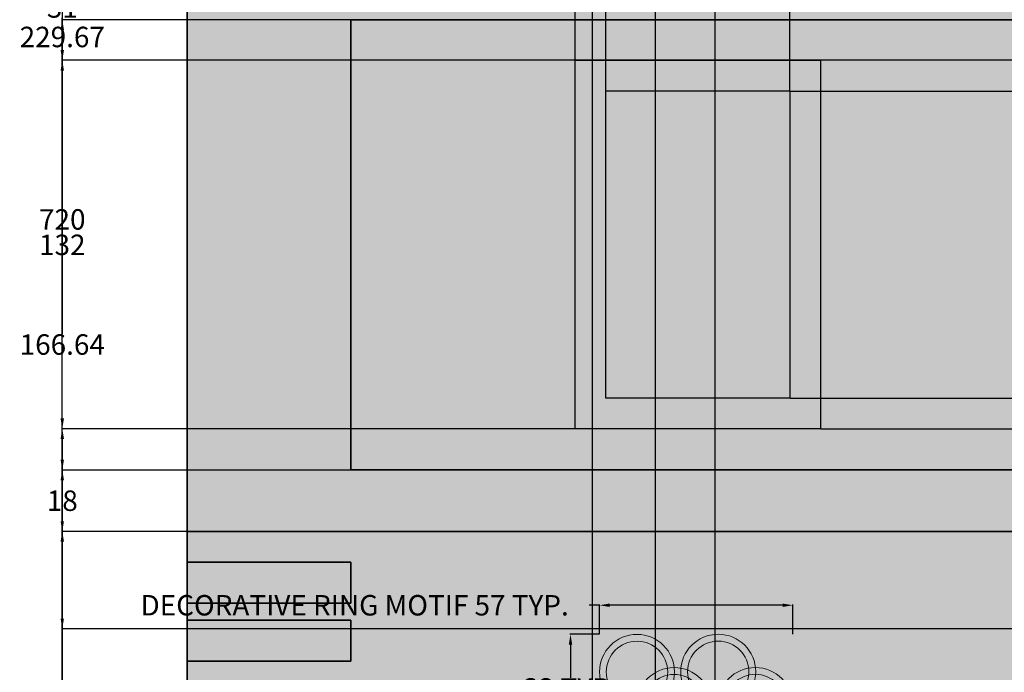
# Model space of a CAD drawing. Units: inches. Extents: x 126 to 726, y 86 to 888.
# Tile 6 of 13: x 137 to 426, y 354 to 546. Entities that reach past the tile are written whole.
import ezdxf

# ---------------------------------------------------------------- set-up
doc = ezdxf.new("R2010")
doc.units = ezdxf.units.IN
doc.header["$MEASUREMENT"] = 0
for name, color, linetype, lineweight in [('A-ANNO-DIMS', 2, 'Continuous', 18), ('A-ELEV', 7, 'Continuous', 35), ('A-ELEV-DECO', 7, 'Continuous', 18), ('A-ELEV-PATT', 8, 'Continuous', 13), ('A-GLAZ', 4, 'Continuous', 25)]:
    doc.layers.add(name, color=color, linetype=linetype, lineweight=lineweight)
doc.styles.get("Standard").update_dxf_attribs({"font": 'arial.ttf'})
doc.dimstyles.get("Standard").update_dxf_attribs({"dimtxt": 6, "dimasz": 3, "dimexe": 0.18, "dimexo": 0.0625, "dimgap": 0.09, "dimtad": 0, "dimtih": 1, "dimtoh": 1, "dimdec": 0, "dimzin": 0, "dimdsep": 46, "dimlunit": 3, "dimtxsty": 'Standard', "dimcen": 0.09, "dimadec": 0, "dimazin": 0, "dimtfac": 1, "dimtdec": 0, "dimtofl": 0, "dimtmove": 0, "dimatfit": 3, "dimfxl": 1, "dimtolj": 1, "dimtzin": 0, "dimarcsym": 0})

# ---------------------------------------------------------------- blocks, each defined once
blk = doc.blocks.new('FACADE-STRIP')
for p, q in [((0, 0), (0, 12)), ((0, 12), (48, 12)), ((0, 0), (48, 0))]:
    blk.add_line(p, q)
blk = doc.blocks.new('WIN-FRAME')
for points in [[(72, 0), (0, 0), (0, 108), (72, 108)], [(63, 9), (9, 9), (9, 99), (63, 99)]]:
    blk.add_lwpolyline(points, close=True)
blk = doc.blocks.new('MOTIF-RINGS')
for centre, radius in [((34.81, 20.77), 11), ((11, 20.74), 11), ((11, 20.74), 9), ((34.81, 20.77), 9), ((21.88, 11), 11), ((45.69, 11.03), 11), ((21.88, 11), 9), ((45.69, 11.03), 9)]:
    blk.add_circle(centre, radius)
blk = doc.blocks.new('*D9')
at = {"layer": 'A-ANNO-DIMS', "color": 0, "lineweight": -2, "transparency": 16777216}
for p, q in [((306.84, 373.93), (303.84, 373.93)), ((306.84, 365.49), (306.84, 374.11)), ((360.53, 373.93), (309.84, 373.93)), ((363.53, 365.49), (363.53, 374.11))]:
    blk.add_line(p, q, dxfattribs=at)
at = {"layer": 'A-ANNO-DIMS', "color": 0, "transparency": 16777216}
for points in [[(309.84, 374.43), (309.84, 373.43), (306.84, 373.93)], [(360.53, 374.43), (360.53, 373.43), (363.53, 373.93)]]:
    blk.add_solid(points, dxfattribs=at)
at = {"layer": 'Defpoints', "color": 0, "transparency": 16777216}
for p in [(306.84, 373.93), (306.84, 365.42), (363.53, 365.42)]:
    blk.add_point(p, dxfattribs=at)
at = {"layer": 'A-ANNO-DIMS', "color": 0, "transparency": 16777216, "insert": (235.05, 373.93), "char_height": 6, "attachment_point": 5}
blk.add_mtext('\\A1;DECORATIVE RING MOTIF 57 TYP.', dxfattribs=at)
blk = doc.blocks.new('*D10')
at = {"layer": 'A-ANNO-DIMS', "color": 0, "lineweight": -2, "transparency": 16777216}
for p, q in [((306.78, 365.42), (298.16, 365.42)), ((298.34, 362.42), (298.34, 352.7)), ((298.34, 336.66), (298.34, 346.38)), ((306.78, 333.66), (298.16, 333.66))]:
    blk.add_line(p, q, dxfattribs=at)
at = {"layer": 'A-ANNO-DIMS', "color": 0, "transparency": 16777216}
for points in [[(297.84, 362.42), (298.84, 362.42), (298.34, 365.42)], [(297.84, 336.66), (298.84, 336.66), (298.34, 333.66)]]:
    blk.add_solid(points, dxfattribs=at)
at = {"layer": 'Defpoints', "color": 0, "transparency": 16777216}
for p in [(306.84, 365.42), (298.34, 333.66), (306.84, 333.66)]:
    blk.add_point(p, dxfattribs=at)
at = {"layer": 'A-ANNO-DIMS', "color": 0, "transparency": 16777216, "insert": (298.34, 349.54), "char_height": 6, "attachment_point": 5}
blk.add_mtext('\\A1;32 TYP.', dxfattribs=at)
blk = doc.blocks.new('*D13')
at = {"layer": 'A-ANNO-DIMS', "color": 0, "lineweight": -2, "transparency": 16777216}
for p, q in [((665.97, 642.98), (665.97, 90.21)), ((185.97, 126.98), (185.97, 90.21)), ((188.97, 90.39), (419.15, 90.39)), ((662.97, 90.39), (432.8, 90.39))]:
    blk.add_line(p, q, dxfattribs=at)
at = {"layer": 'A-ANNO-DIMS', "color": 0, "transparency": 16777216}
for points in [[(188.97, 90.89), (188.97, 89.89), (185.97, 90.39)], [(662.97, 90.89), (662.97, 89.89), (665.97, 90.39)]]:
    blk.add_solid(points, dxfattribs=at)
at = {"layer": 'Defpoints', "color": 0, "transparency": 16777216}
for p in [(665.97, 643.04), (185.97, 127.04), (665.97, 90.39)]:
    blk.add_point(p, dxfattribs=at)
at = {"layer": 'A-ANNO-DIMS', "color": 0, "transparency": 16777216, "insert": (425.97, 90.39), "char_height": 6, "attachment_point": 5}
blk.add_mtext('\\A1;480', dxfattribs=at)
blk = doc.blocks.new('*D14')
at = {"layer": 'A-ANNO-DIMS', "color": 0, "lineweight": -2, "transparency": 16777216}
for p, q in [((185.91, 847.04), (149.14, 847.04)), ((149.32, 844.04), (149.32, 490.2)), ((149.32, 130.04), (149.32, 483.89)), ((185.91, 127.04), (149.14, 127.04))]:
    blk.add_line(p, q, dxfattribs=at)
at = {"layer": 'A-ANNO-DIMS', "color": 0, "transparency": 16777216}
for points in [[(148.82, 844.04), (149.82, 844.04), (149.32, 847.04)], [(148.82, 130.04), (149.82, 130.04), (149.32, 127.04)]]:
    blk.add_solid(points, dxfattribs=at)
at = {"layer": 'Defpoints', "color": 0, "transparency": 16777216}
for p in [(149.32, 847.04), (185.97, 847.04), (185.97, 127.04)]:
    blk.add_point(p, dxfattribs=at)
at = {"layer": 'A-ANNO-DIMS', "color": 0, "transparency": 16777216, "insert": (149.32, 487.04), "char_height": 6, "attachment_point": 5}
blk.add_mtext('\\A1;720', dxfattribs=at)
blk = doc.blocks.new('*D16')
at = {"layer": 'A-ANNO-DIMS', "color": 0, "lineweight": -2, "transparency": 16777216}
for p, q in [((299.6, 425.68), (149.14, 425.68)), ((149.32, 422.68), (149.32, 313.79)), ((149.32, 198.59), (149.32, 307.48)), ((299.6, 195.59), (149.14, 195.59))]:
    blk.add_line(p, q, dxfattribs=at)
at = {"layer": 'A-ANNO-DIMS', "color": 0, "transparency": 16777216}
for points in [[(148.82, 422.68), (149.82, 422.68), (149.32, 425.68)], [(148.82, 198.59), (149.82, 198.59), (149.32, 195.59)]]:
    blk.add_solid(points, dxfattribs=at)
at = {"layer": 'Defpoints', "color": 0, "transparency": 16777216}
for p in [(149.32, 425.68), (299.67, 425.68), (299.67, 195.59)]:
    blk.add_point(p, dxfattribs=at)
at = {"layer": 'A-ANNO-DIMS', "color": 0, "transparency": 16777216, "insert": (149.32, 310.64), "char_height": 6, "attachment_point": 5}
blk.add_mtext('\\A1;230.1', dxfattribs=at)
blk = doc.blocks.new('*D17')
at = {"layer": 'A-ANNO-DIMS', "color": 0, "lineweight": -2, "transparency": 16777216}
for p, q in [((299.26, 655.35), (149.14, 655.35)), ((149.32, 652.35), (149.32, 543.67)), ((149.32, 428.68), (149.32, 537.37)), ((299.6, 425.68), (149.14, 425.68))]:
    blk.add_line(p, q, dxfattribs=at)
at = {"layer": 'A-ANNO-DIMS', "color": 0, "transparency": 16777216}
for points in [[(148.82, 652.35), (149.82, 652.35), (149.32, 655.35)], [(148.82, 428.68), (149.82, 428.68), (149.32, 425.68)]]:
    blk.add_solid(points, dxfattribs=at)
at = {"layer": 'Defpoints', "color": 0, "transparency": 16777216}
for p in [(149.32, 655.35), (299.32, 655.35), (299.67, 425.68)]:
    blk.add_point(p, dxfattribs=at)
at = {"layer": 'A-ANNO-DIMS', "color": 0, "transparency": 16777216, "insert": (149.32, 540.52), "char_height": 6, "attachment_point": 5}
blk.add_mtext('\\A1;229.67', dxfattribs=at)
blk = doc.blocks.new('*D18')
at = {"layer": 'A-ANNO-DIMS', "color": 0, "lineweight": -2, "transparency": 16777216}
for p, q in [((431.28, 395.58), (149.14, 395.58)), ((149.32, 392.58), (149.32, 264.47)), ((149.32, 130.04), (149.32, 258.16)), ((185.91, 127.04), (149.14, 127.04))]:
    blk.add_line(p, q, dxfattribs=at)
at = {"layer": 'A-ANNO-DIMS', "color": 0, "transparency": 16777216}
for points in [[(148.82, 392.58), (149.82, 392.58), (149.32, 395.58)], [(148.82, 130.04), (149.82, 130.04), (149.32, 127.04)]]:
    blk.add_solid(points, dxfattribs=at)
at = {"layer": 'Defpoints', "color": 0, "transparency": 16777216}
for p in [(149.32, 395.58), (431.34, 395.58), (185.97, 127.04)]:
    blk.add_point(p, dxfattribs=at)
at = {"layer": 'A-ANNO-DIMS', "color": 0, "transparency": 16777216, "insert": (149.32, 261.31), "char_height": 6, "attachment_point": 5}
blk.add_mtext('\\A1;268.54', dxfattribs=at)
blk = doc.blocks.new('*D19')
at = {"layer": 'A-ANNO-DIMS', "color": 0, "lineweight": -2, "transparency": 16777216}
for p, q in [((233.91, 413.58), (149.14, 413.58)), ((149.32, 410.58), (149.32, 407.74)), ((149.32, 398.58), (149.32, 401.43)), ((431.28, 395.58), (149.14, 395.58))]:
    blk.add_line(p, q, dxfattribs=at)
at = {"layer": 'A-ANNO-DIMS', "color": 0, "transparency": 16777216}
for points in [[(148.82, 410.58), (149.82, 410.58), (149.32, 413.58)], [(148.82, 398.58), (149.82, 398.58), (149.32, 395.58)]]:
    blk.add_solid(points, dxfattribs=at)
at = {"layer": 'Defpoints', "color": 0, "transparency": 16777216}
for p in [(149.32, 413.58), (233.97, 413.58), (431.34, 395.58)]:
    blk.add_point(p, dxfattribs=at)
at = {"layer": 'A-ANNO-DIMS', "color": 0, "transparency": 16777216, "insert": (149.32, 404.58), "char_height": 6, "attachment_point": 5}
blk.add_mtext('\\A1;18', dxfattribs=at)
blk = doc.blocks.new('*D20')
at = {"layer": 'A-ANNO-DIMS', "color": 0, "lineweight": -2, "transparency": 16777216}
for p, q in [((233.91, 545.58), (149.14, 545.58)), ((149.32, 542.58), (149.32, 482.74)), ((149.32, 416.58), (149.32, 476.43)), ((233.91, 413.58), (149.14, 413.58))]:
    blk.add_line(p, q, dxfattribs=at)
at = {"layer": 'A-ANNO-DIMS', "color": 0, "transparency": 16777216}
for points in [[(148.82, 542.58), (149.82, 542.58), (149.32, 545.58)], [(148.82, 416.58), (149.82, 416.58), (149.32, 413.58)]]:
    blk.add_solid(points, dxfattribs=at)
at = {"layer": 'Defpoints', "color": 0, "transparency": 16777216}
for p in [(149.32, 545.58), (233.97, 545.58), (233.97, 413.58)]:
    blk.add_point(p, dxfattribs=at)
at = {"layer": 'A-ANNO-DIMS', "color": 0, "transparency": 16777216, "insert": (149.32, 479.58), "char_height": 6, "attachment_point": 5}
blk.add_mtext('\\A1;132', dxfattribs=at)
blk = doc.blocks.new('*D32')
at = {"layer": 'A-ANNO-DIMS', "color": 0, "lineweight": -2, "transparency": 16777216}
for p, q in [((299.67, 533.75), (299.67, 883.87)), ((302.67, 883.69), (305.67, 883.69)), ((308.67, 524.75), (308.67, 883.87)), ((308.67, 883.69), (311.67, 883.69))]:
    blk.add_line(p, q, dxfattribs=at)
at = {"layer": 'A-ANNO-DIMS', "color": 0, "transparency": 16777216}
for points in [[(302.67, 884.19), (302.67, 883.19), (299.67, 883.69)], [(305.67, 884.19), (305.67, 883.19), (308.67, 883.69)]]:
    blk.add_solid(points, dxfattribs=at)
at = {"layer": 'Defpoints', "color": 0, "transparency": 16777216}
for p in [(308.67, 883.69), (299.67, 533.68), (308.67, 524.68)]:
    blk.add_point(p, dxfattribs=at)
at = {"layer": 'A-ANNO-DIMS', "color": 0, "transparency": 16777216, "insert": (313.73, 883.69), "char_height": 6, "attachment_point": 5}
blk.add_mtext('\\A1;9', dxfattribs=at)
blk = doc.blocks.new('*D33')
at = {"layer": 'A-ANNO-DIMS', "color": 0, "lineweight": -2, "transparency": 16777216}
for p, q in [((308.67, 524.75), (308.67, 883.87)), ((311.67, 883.69), (331.29, 883.69)), ((359.67, 883.69), (340.04, 883.69)), ((362.67, 524.75), (362.67, 883.87))]:
    blk.add_line(p, q, dxfattribs=at)
at = {"layer": 'A-ANNO-DIMS', "color": 0, "transparency": 16777216}
for points in [[(311.67, 884.19), (311.67, 883.19), (308.67, 883.69)], [(359.67, 884.19), (359.67, 883.19), (362.67, 883.69)]]:
    blk.add_solid(points, dxfattribs=at)
at = {"layer": 'Defpoints', "color": 0, "transparency": 16777216}
for p in [(362.67, 883.69), (308.67, 524.68), (362.67, 524.68)]:
    blk.add_point(p, dxfattribs=at)
at = {"layer": 'A-ANNO-DIMS', "color": 0, "transparency": 16777216, "insert": (335.67, 883.69), "char_height": 6, "attachment_point": 5}
blk.add_mtext('\\A1;54', dxfattribs=at)
blk = doc.blocks.new('*D34')
at = {"layer": 'A-ANNO-DIMS', "color": 0, "lineweight": -2, "transparency": 16777216}
for p, q in [((362.73, 524.68), (702.8, 524.68)), ((702.62, 521.68), (702.62, 482.84)), ((702.62, 437.68), (702.62, 476.53)), ((362.73, 434.68), (702.8, 434.68))]:
    blk.add_line(p, q, dxfattribs=at)
at = {"layer": 'A-ANNO-DIMS', "color": 0, "transparency": 16777216}
for points in [[(702.12, 521.68), (703.12, 521.68), (702.62, 524.68)], [(702.12, 437.68), (703.12, 437.68), (702.62, 434.68)]]:
    blk.add_solid(points, dxfattribs=at)
at = {"layer": 'Defpoints', "color": 0, "transparency": 16777216}
for p in [(362.67, 524.68), (702.62, 524.68), (362.67, 434.68)]:
    blk.add_point(p, dxfattribs=at)
at = {"layer": 'A-ANNO-DIMS', "color": 0, "transparency": 16777216, "insert": (702.62, 479.68), "char_height": 6, "attachment_point": 5}
blk.add_mtext('\\A1;90', dxfattribs=at)
blk = doc.blocks.new('*D35')
at = {"layer": 'A-ANNO-DIMS', "color": 0, "lineweight": -2, "transparency": 16777216}
for p, q in [((702.624909, 437.684516), (702.624909, 440.684516)), ((362.728342, 434.684516), (702.804909, 434.684516)), ((371.728342, 425.684516), (702.804909, 425.684516)), ((702.624909, 422.684516), (702.624909, 419.684516))]:
    blk.add_line(p, q, dxfattribs=at)
at = {"layer": 'A-ANNO-DIMS', "color": 0, "transparency": 16777216}
for points in [[(702.124909, 437.684516), (703.124909, 437.684516), (702.624909, 434.684516)], [(702.124909, 422.684516), (703.124909, 422.684516), (702.624909, 425.684516)]]:
    blk.add_solid(points, dxfattribs=at)
at = {"layer": 'Defpoints', "color": 0, "transparency": 16777216}
for p in [(362.665842, 434.684516), (702.624909, 434.684516), (371.665842, 425.684516)]:
    blk.add_point(p, dxfattribs=at)
at = {"layer": 'A-ANNO-DIMS', "color": 0, "transparency": 16777216, "insert": (702.624909, 430.184516), "char_height": 6, "attachment_point": 5}
blk.add_mtext('\\A1;9', dxfattribs=at)
blk = doc.blocks.new('*D38')
at = {"layer": 'A-ANNO-DIMS', "color": 0, "lineweight": -2, "transparency": 16777216}
for p, q in [((304.8, 168.3), (304.8, 883.87)), ((307.8, 883.69), (320.3, 883.69)), ((323.3, 174.45), (323.3, 883.87)), ((323.3, 883.69), (326.3, 883.69))]:
    blk.add_line(p, q, dxfattribs=at)
at = {"layer": 'A-ANNO-DIMS', "color": 0, "transparency": 16777216}
for points in [[(307.8, 884.19), (307.8, 883.19), (304.8, 883.69)], [(320.3, 884.19), (320.3, 883.19), (323.3, 883.69)]]:
    blk.add_solid(points, dxfattribs=at)
at = {"layer": 'Defpoints', "color": 0, "transparency": 16777216}
for p in [(323.3, 883.69), (323.3, 174.39), (304.8, 168.24)]:
    blk.add_point(p, dxfattribs=at)
at = {"layer": 'A-ANNO-DIMS', "color": 0, "transparency": 16777216, "insert": (338.59, 883.69), "char_height": 6, "attachment_point": 5}
blk.add_mtext('\\A1;18.505', dxfattribs=at)
blk = doc.blocks.new('*D39')
at = {"layer": 'A-ANNO-DIMS', "color": 0, "lineweight": -2, "transparency": 16777216}
for p, q in [((323.3, 174.45), (323.3, 883.87)), ((326.3, 883.69), (337.74, 883.69)), ((340.74, 168.3), (340.74, 883.87)), ((340.74, 883.69), (343.74, 883.69))]:
    blk.add_line(p, q, dxfattribs=at)
at = {"layer": 'A-ANNO-DIMS', "color": 0, "transparency": 16777216}
for points in [[(326.3, 884.19), (326.3, 883.19), (323.3, 883.69)], [(337.74, 884.19), (337.74, 883.19), (340.74, 883.69)]]:
    blk.add_solid(points, dxfattribs=at)
at = {"layer": 'Defpoints', "color": 0, "transparency": 16777216}
for p in [(340.74, 883.69), (323.3, 174.39), (340.74, 168.24)]:
    blk.add_point(p, dxfattribs=at)
at = {"layer": 'A-ANNO-DIMS', "color": 0, "transparency": 16777216, "insert": (355.99, 883.69), "char_height": 6, "attachment_point": 5}
blk.add_mtext('\\A1;17.434', dxfattribs=at)
blk = doc.blocks.new('*D58')
at = {"layer": 'A-ANNO-DIMS', "color": 0, "lineweight": -2, "transparency": 16777216}
for p, q in [((485.91, 533.68), (149.14, 533.68)), ((149.32, 530.68), (149.32, 453.52)), ((149.32, 370.04), (149.32, 447.21)), ((485.91, 367.04), (149.14, 367.04))]:
    blk.add_line(p, q, dxfattribs=at)
at = {"layer": 'A-ANNO-DIMS', "color": 0, "transparency": 16777216}
for points in [[(148.82, 530.68), (149.82, 530.68), (149.32, 533.68)], [(148.82, 370.04), (149.82, 370.04), (149.32, 367.04)]]:
    blk.add_solid(points, dxfattribs=at)
at = {"layer": 'Defpoints', "color": 0, "transparency": 16777216}
for p in [(149.32, 533.68), (485.97, 533.68), (485.97, 367.04)]:
    blk.add_point(p, dxfattribs=at)
at = {"layer": 'A-ANNO-DIMS', "color": 0, "transparency": 16777216, "insert": (149.32, 450.36), "char_height": 6, "attachment_point": 5}
blk.add_mtext('\\A1;166.64', dxfattribs=at)
blk = doc.blocks.new('*D59')
at = {"layer": 'A-ANNO-DIMS', "color": 0, "lineweight": -2, "transparency": 16777216}
for p, q in [((485.91, 564.68), (149.14, 564.68)), ((149.32, 561.68), (149.32, 552.34)), ((149.32, 536.68), (149.32, 546.03)), ((485.91, 533.68), (149.14, 533.68))]:
    blk.add_line(p, q, dxfattribs=at)
at = {"layer": 'A-ANNO-DIMS', "color": 0, "transparency": 16777216}
for points in [[(148.82, 561.68), (149.82, 561.68), (149.32, 564.68)], [(148.82, 536.68), (149.82, 536.68), (149.32, 533.68)]]:
    blk.add_solid(points, dxfattribs=at)
at = {"layer": 'Defpoints', "color": 0, "transparency": 16777216}
for p in [(149.32, 564.68), (485.97, 564.68), (485.97, 533.68)]:
    blk.add_point(p, dxfattribs=at)
at = {"layer": 'A-ANNO-DIMS', "color": 0, "transparency": 16777216, "insert": (149.32, 549.18), "char_height": 6, "attachment_point": 5}
blk.add_mtext('\\A1;31', dxfattribs=at)

msp = doc.modelspace()

# ---------------------------------------------------------------- hatches: boundary and pattern name
at = {"layer": 'A-ELEV-PATT'}
h = msp.add_hatch(color=256, dxfattribs=at)
h.dxf.hatch_style = 1
h.paths.add_polyline_path([(233.9749, 545.5846), (431.3386, 545.5846), (431.3386, 563.5846), (185.9749, 563.5846), (185.9749, 395.5846), (431.3386, 395.5846), (431.3386, 413.5846), (233.9749, 413.5846)])
h.paths.add_polyline_path([(233.9749, 835.0424), (485.9749, 835.0424), (605.9749, 835.0424), (605.9749, 847.0424), (485.9749, 847.0424), (185.9749, 847.0424), (185.9749, 606.5846), (233.9749, 606.5846)])
h.paths.add_polyline_path([(233.9749, 597.5846), (185.9749, 597.5846), (185.9749, 585.5846), (233.9749, 585.5846)])
h.paths.add_polyline_path([(233.9749, 580.5846), (185.9749, 580.5846), (185.9749, 568.5846), (233.9749, 568.5846)])
h = msp.add_hatch(color=256, dxfattribs=at)
h.dxf.hatch_style = 1
h.paths.add_polyline_path([(437.9749, 499.1312), (485.9749, 499.1312), (485.9749, 501.4423), (437.9749, 501.4423), (437.9749, 513.4423), (485.9749, 513.4423), (485.9749, 515.7534), (437.9749, 515.7534), (437.9749, 527.7534), (485.9749, 527.7534), (485.9749, 530.0646), (437.9749, 530.0646), (437.9749, 542.0646), (485.9749, 542.0646), (485.9749, 544.3757), (437.9749, 544.3757), (437.9749, 556.3757), (485.9749, 556.3757), (485.9749, 558.6868), (437.9749, 558.6868), (437.9749, 570.6868), (485.9749, 570.6868), (485.9749, 572.9979), (437.9749, 572.9979), (437.9749, 584.9979), (485.9749, 584.9979), (485.9749, 587.309), (437.9749, 587.309), (437.9749, 595.0424), (429.9749, 595.0424), (429.9749, 607.0424), (437.9749, 607.0424), (437.9749, 615.9312), (437.9749, 630.2423), (437.9749, 642.2423), (485.9749, 642.2423), (485.9749, 644.5534), (437.9749, 644.5534), (437.9749, 656.5534), (485.9749, 656.5534), (485.9749, 658.8645), (437.9749, 658.8645), (437.9749, 670.8645), (485.9749, 670.8645), (485.9749, 673.1757), (437.9749, 673.1757), (437.9749, 685.1757), (485.9749, 685.1757), (485.9749, 687.4868), (437.9749, 687.4868), (437.9749, 699.4868), (485.9749, 699.4868), (485.9749, 701.7979), (437.9749, 701.7979), (437.9749, 713.7979), (485.9749, 713.7979), (485.9749, 716.109), (437.9749, 716.109), (437.9749, 728.109), (485.9749, 728.109), (485.9749, 730.4201), (437.9749, 730.4201), (437.9749, 742.4201), (485.9749, 742.4201), (485.9749, 744.7312), (437.9749, 744.7312), (437.9749, 756.7312), (485.9749, 756.7312), (485.9749, 759.0423), (437.9749, 759.0423), (437.9749, 771.0423), (485.9749, 771.0423), (485.9749, 773.3534), (437.9749, 773.3534), (437.9749, 785.3534), (485.9749, 785.3534), (485.9749, 787.6645), (437.9749, 787.6645), (437.9749, 799.6645), (485.9749, 799.6645), (485.9749, 801.9756), (437.9749, 801.9756), (437.9749, 811.2868), (485.9749, 811.2868), (485.9749, 813.9756), (437.9749, 813.9756), (437.9749, 825.9756), (485.9749, 825.9756), (485.9749, 835.0424), (233.9749, 835.0424), (233.9749, 606.5846), (185.9749, 606.5846), (185.9749, 597.5846), (233.9749, 597.5846), (233.9749, 585.5846), (185.9749, 585.5846), (185.9749, 580.5846), (233.9749, 580.5846), (233.9749, 568.5846), (185.9749, 568.5846), (185.9749, 563.5846), (431.3386, 563.5846), (431.3386, 545.5846), (233.9749, 545.5846), (233.9749, 413.5846), (431.3386, 413.5846), (431.3386, 395.5846), (185.9749, 395.5846), (185.9749, 386.5846), (233.9749, 386.5846), (233.9749, 374.5846), (185.9749, 374.5846), (185.9749, 369.5846), (233.9749, 369.5846), (233.9749, 357.5846), (185.9749, 357.5846), (185.9749, 352.5846), (233.9749, 352.5846), (233.9749, 340.5846), (185.9749, 340.5846), (185.9749, 331.5846), (233.9749, 331.5846), (233.9749, 127.0424), (485.9749, 127.0424), (485.9749, 129.3535), (437.9749, 129.3535), (437.9749, 141.3535), (485.9749, 141.3535), (485.9749, 143.6646), (437.9749, 143.6646), (437.9749, 155.6646), (485.9749, 155.6646), (485.9749, 157.9757), (437.9749, 157.9757), (437.9749, 169.9757), (485.9749, 169.9757), (485.9749, 172.2868), (437.9749, 172.2868), (437.9749, 184.2868), (485.9749, 184.2868), (485.9749, 186.5979), (437.9749, 186.5979), (437.9749, 198.5979), (485.9749, 198.5979), (485.9749, 200.909), (437.9749, 200.909), (437.9749, 212.909), (485.9749, 212.909), (485.9749, 215.2201), (437.9749, 215.2201), (437.9749, 227.2201), (485.9749, 227.2201), (485.9749, 229.5312), (437.9749, 229.5312), (437.9749, 241.5312), (485.9749, 241.5312), (485.9749, 243.8424), (437.9749, 243.8424), (437.9749, 255.8424), (485.9749, 255.8424), (485.9749, 258.1535), (437.9749, 258.1535), (437.9749, 270.1535), (485.9749, 270.1535), (485.9749, 272.4646), (437.9749, 272.4646), (437.9749, 284.4646), (485.9749, 284.4646), (485.9749, 286.7757), (437.9749, 286.7757), (437.9749, 298.7757), (485.9749, 298.7757), (485.9749, 301.0868), (437.9749, 301.0868), (437.9749, 313.0868), (485.9749, 313.0868), (485.9749, 315.3979), (437.9749, 315.3979), (437.9749, 327.3979), (485.9749, 327.3979), (485.9749, 329.709), (437.9749, 329.709), (437.9749, 341.709), (485.9749, 341.709), (485.9749, 344.0201), (437.9749, 344.0201), (437.9749, 355.0424), (429.9749, 355.0424), (429.9749, 367.0424), (437.9749, 367.0424), (437.9749, 372.6423), (437.9749, 386.9535), (437.9749, 401.2646), (437.9749, 413.2646), (485.9749, 413.2646), (485.9749, 415.5757), (437.9749, 415.5757), (437.9749, 427.5757), (485.9749, 427.5757), (485.9749, 429.8868), (437.9749, 429.8868), (437.9749, 441.8868), (485.9749, 441.8868), (485.9749, 444.1979), (437.9749, 444.1979), (437.9749, 456.1979), (485.9749, 456.1979), (485.9749, 458.509), (437.9749, 458.509), (437.9749, 470.509), (485.9749, 470.509), (485.9749, 472.8201), (437.9749, 472.8201), (437.9749, 484.8201), (485.9749, 484.8201), (485.9749, 487.1312), (437.9749, 487.1312)])
h.paths.add_polyline_path([(299.6658, 533.6845), (371.6658, 533.6845), (371.6658, 425.6845), (299.6658, 425.6845)], flags=16)
h.paths.add_polyline_path([(308.6658, 524.6845), (362.6658, 524.6845), (362.6658, 434.6845), (308.6658, 434.6845)], flags=0)
h.paths.add_polyline_path([(317.7956, 603.3211, -0.4129833), (306.8418, 614.321, -0.94403766), (328.769, 615.5845, -0.04423165), (330.7031, 615.4048, -0.89973713), (352.5798, 615.6161, -0.4129833), (363.5336, 604.6162, -0.94403766), (341.6064, 603.3528, -0.04423165), (339.6723, 603.5324, -0.89973713)], flags=16)
h.paths.add_polyline_path([(319.7228, 604.5846, -0.02633223), (319.7726, 605.5306, -0.47905713), (308.8418, 614.321, -1), (326.8418, 614.321, -0.02633223), (326.7919, 613.375, -0.17413188), (332.826, 612.5948, -0.04918553), (332.6526, 614.3527, -1), (350.6526, 614.3527, -0.02633223), (350.6028, 613.4067, -0.47905713), (361.5336, 604.6162, -1), (343.5336, 604.6162, -0.02633223), (343.5834, 605.5622, -0.17413188), (337.5494, 606.3424, -0.04918553), (337.7228, 604.5846, -1)], flags=0)
h.paths.add_polyline_path([(328.769, 355.6561, -0.04423165), (330.7031, 355.4765, -0.89973713), (352.5798, 355.6878, -0.4129833), (363.5336, 344.6879, -0.94403766), (341.6064, 343.4244, -0.04423165), (339.6723, 343.604, -0.89973713), (317.7956, 343.3927, -0.4129833), (306.8418, 354.3926, -0.94403766)], flags=16)
h.paths.add_polyline_path([(326.8418, 354.3926, -0.02633223), (326.7919, 353.4466, -0.17413188), (332.826, 352.6664, -0.04918553), (332.6526, 354.4243, -1), (350.6526, 354.4243, -0.02633223), (350.6028, 353.4783, -0.47905713), (361.5336, 344.6879, -1), (343.5336, 344.6879, -0.02633223), (343.5834, 345.6339, -0.17413188), (337.5494, 346.4141, -0.04918553), (337.7228, 344.6562, -1), (319.7228, 344.6562, -0.02633223), (319.7726, 345.6022, -0.47905713), (308.8418, 354.3926, -1)], flags=0)
h.paths.add_polyline_path([(299.3189, 655.3527), (299.3189, 763.3527), (371.3189, 763.3527), (371.3189, 655.3527)], flags=16)
h.paths.add_polyline_path([(308.3189, 664.3527), (308.3189, 754.3527), (362.3189, 754.3527), (362.3189, 664.3527)], flags=0)
h.paths.add_polyline_path([(299.6658, 303.5875), (371.6658, 303.5875), (371.6658, 195.5875), (299.6658, 195.5875)], flags=16)
h.paths.add_polyline_path([(308.6658, 294.5875), (362.6658, 294.5875), (362.6658, 204.5875), (308.6658, 204.5875)], flags=0)
h.paths.add_polyline_path([(326.3038, 177.3867), (346.055, 177.3867, -0.41421356), (349.055, 174.3867), (349.055, 171.2378), (363.489, 171.2378, -0.41421356), (366.489, 168.2378), (366.489, 159.7133, -0.41421356), (363.489, 156.7133), (343.7379, 156.7133, -0.41421356), (340.7379, 159.7133), (340.7379, 162.8622), (330.5504, 162.8622), (330.5504, 159.7133, -0.41421356), (327.5504, 156.7133), (307.7992, 156.7133, -0.41421356), (304.7992, 159.7133), (304.7992, 168.2378, -0.41421356), (307.7992, 171.2378), (323.3038, 171.2378), (323.3038, 174.3867, -0.41421356)], flags=16)
h.paths.add_polyline_path([(326.3038, 175.3867), (346.055, 175.3867, -0.41421356), (347.055, 174.3867), (347.055, 169.2378), (363.489, 169.2378, -0.41421356), (364.489, 168.2378), (364.489, 159.7133, -0.41421356), (363.489, 158.7133), (343.7379, 158.7133, -0.41421356), (342.7379, 159.7133), (342.7379, 164.8622), (328.5504, 164.8622), (328.5504, 159.7133, -0.41421356), (327.5504, 158.7133), (307.7992, 158.7133, -0.41421356), (306.7992, 159.7133), (306.7992, 168.2378, -0.41421356), (307.7992, 169.2378), (325.3038, 169.2378), (325.3038, 174.3867, -0.41421356)], flags=0)
h = msp.add_hatch(dxfattribs=at)
h.set_pattern_fill('GRAVEL', color=256, scale=40)
h.paths.add_polyline_path([(437.9749, 642.2423), (485.9749, 642.2423), (485.9749, 644.5534), (437.9749, 644.5534), (437.9749, 656.5534), (485.9749, 656.5534), (485.9749, 658.8645), (437.9749, 658.8645), (437.9749, 670.8645), (485.9749, 670.8645), (485.9749, 673.1757), (437.9749, 673.1757), (437.9749, 685.1757), (485.9749, 685.1757), (485.9749, 687.4868), (437.9749, 687.4868), (437.9749, 699.4868), (485.9749, 699.4868), (485.9749, 701.7979), (437.9749, 701.7979), (437.9749, 713.7979), (485.9749, 713.7979), (485.9749, 716.109), (437.9749, 716.109), (437.9749, 728.109), (485.9749, 728.109), (485.9749, 730.4201), (437.9749, 730.4201), (437.9749, 742.4201), (485.9749, 742.4201), (485.9749, 744.7312), (437.9749, 744.7312), (437.9749, 756.7312), (485.9749, 756.7312), (485.9749, 759.0423), (437.9749, 759.0423), (437.9749, 771.0423), (485.9749, 771.0423), (485.9749, 773.3534), (437.9749, 773.3534), (437.9749, 785.3534), (485.9749, 785.3534), (485.9749, 787.6645), (437.9749, 787.6645), (437.9749, 799.6645), (485.9749, 799.6645), (485.9749, 801.9756), (437.9749, 801.9756), (437.9749, 811.2868), (485.9749, 811.2868), (485.9749, 813.9756), (437.9749, 813.9756), (437.9749, 825.9756), (485.9749, 825.9756), (485.9749, 835.0424), (233.9749, 835.0424), (233.9749, 606.5846), (185.9749, 606.5846), (185.9749, 597.5846), (233.9749, 597.5846), (233.9749, 585.5846), (185.9749, 585.5846), (185.9749, 580.5846), (233.9749, 580.5846), (233.9749, 568.5846), (185.9749, 568.5846), (185.9749, 563.5846), (431.3386, 563.5846), (431.3386, 545.5846), (233.9749, 545.5846), (233.9749, 413.5846), (431.3386, 413.5846), (431.3386, 395.5846), (185.9749, 395.5846), (185.9749, 386.5846), (233.9749, 386.5846), (233.9749, 374.5846), (185.9749, 374.5846), (185.9749, 369.5846), (233.9749, 369.5846), (233.9749, 357.5846), (185.9749, 357.5846), (185.9749, 352.5846), (233.9749, 352.5846), (233.9749, 340.5846), (185.9749, 340.5846), (185.9749, 331.5846), (233.9749, 331.5846), (233.9749, 127.0424), (485.9749, 127.0424), (485.9749, 129.3535), (437.9749, 129.3535), (437.9749, 141.3535), (485.9749, 141.3535), (485.9749, 143.6646), (437.9749, 143.6646), (437.9749, 155.6646), (485.9749, 155.6646), (485.9749, 157.9757), (437.9749, 157.9757), (437.9749, 169.9757), (485.9749, 169.9757), (485.9749, 172.2868), (437.9749, 172.2868), (437.9749, 184.2868), (485.9749, 184.2868), (485.9749, 186.5979), (437.9749, 186.5979), (437.9749, 198.5979), (485.9749, 198.5979), (485.9749, 200.909), (437.9749, 200.909), (437.9749, 212.909), (485.9749, 212.909), (485.9749, 215.2201), (437.9749, 215.2201), (437.9749, 227.2201), (485.9749, 227.2201), (485.9749, 229.5312), (437.9749, 229.5312), (437.9749, 241.5312), (485.9749, 241.5312), (485.9749, 243.8424), (437.9749, 243.8424), (437.9749, 255.8424), (485.9749, 255.8424), (485.9749, 258.1535), (437.9749, 258.1535), (437.9749, 270.1535), (485.9749, 270.1535), (485.9749, 272.4646), (437.9749, 272.4646), (437.9749, 284.4646), (485.9749, 284.4646), (485.9749, 286.7757), (437.9749, 286.7757), (437.9749, 298.7757), (485.9749, 298.7757), (485.9749, 301.0868), (437.9749, 301.0868), (437.9749, 313.0868), (485.9749, 313.0868), (485.9749, 315.3979), (437.9749, 315.3979), (437.9749, 327.3979), (485.9749, 327.3979), (485.9749, 329.709), (437.9749, 329.709), (437.9749, 341.709), (485.9749, 341.709), (485.9749, 344.0201), (437.9749, 344.0201), (437.9749, 355.0424), (429.9749, 355.0424), (429.9749, 367.0424), (437.9749, 367.0424), (437.9749, 372.6423), (437.9749, 386.9535), (437.9749, 401.2646), (437.9749, 413.2646), (485.9749, 413.2646), (485.9749, 415.5757), (437.9749, 415.5757), (437.9749, 427.5757), (485.9749, 427.5757), (485.9749, 429.8868), (437.9749, 429.8868), (437.9749, 441.8868), (485.9749, 441.8868), (485.9749, 444.1979), (437.9749, 444.1979), (437.9749, 456.1979), (485.9749, 456.1979), (485.9749, 458.509), (437.9749, 458.509), (437.9749, 470.509), (485.9749, 470.509), (485.9749, 472.8201), (437.9749, 472.8201), (437.9749, 484.8201), (485.9749, 484.8201), (485.9749, 487.1312), (437.9749, 487.1312), (437.9749, 499.1312), (485.9749, 499.1312), (485.9749, 501.4423), (437.9749, 501.4423), (437.9749, 513.4423), (485.9749, 513.4423), (485.9749, 515.7534), (437.9749, 515.7534), (437.9749, 527.7534), (485.9749, 527.7534), (485.9749, 530.0646), (437.9749, 530.0646), (437.9749, 542.0646), (485.9749, 542.0646), (485.9749, 544.3757), (437.9749, 544.3757), (437.9749, 556.3757), (485.9749, 556.3757), (485.9749, 558.6868), (437.9749, 558.6868), (437.9749, 570.6868), (485.9749, 570.6868), (485.9749, 572.9979), (437.9749, 572.9979), (437.9749, 584.9979), (485.9749, 584.9979), (485.9749, 587.309), (437.9749, 587.309), (437.9749, 595.0424), (429.9749, 595.0424), (429.9749, 607.0424), (437.9749, 607.0424), (437.9749, 615.9312), (437.9749, 630.2423)])
h.paths.add_polyline_path([(371.3189, 655.3527), (299.3189, 655.3527), (299.3189, 763.3527), (371.3189, 763.3527)], flags=16)
h.paths.add_polyline_path([(363.5336, 604.6162, -0.94403766), (341.6064, 603.3528, -0.04423165), (339.6723, 603.5324, -0.89973713), (317.7956, 603.3211, -0.4129833), (306.8418, 614.321, -0.94403766), (328.769, 615.5845, -0.04423165), (330.7031, 615.4048, -0.89973713), (352.5798, 615.6161, -0.4129833)], flags=16)
h.paths.add_polyline_path([(361.5336, 604.6162, -1), (343.5336, 604.6162, -0.02633223), (343.5834, 605.5622, -0.17413188), (337.5494, 606.3424, -0.04918553), (337.7228, 604.5846, -1), (319.7228, 604.5846, -0.02633223), (319.7726, 605.5306, -0.47905713), (308.8418, 614.321, -1), (326.8418, 614.321, -0.02633223), (326.7919, 613.375, -0.17413188), (332.826, 612.5948, -0.04918553), (332.6526, 614.3527, -1), (350.6526, 614.3527, -0.02633223), (350.6028, 613.4067, -0.47905713)], flags=0)
h.paths.add_polyline_path([(362.3189, 664.3527), (308.3189, 664.3527), (308.3189, 754.3527), (362.3189, 754.3527)], flags=0)
h.paths.add_polyline_path([(371.6658, 533.6845), (371.6658, 425.6845), (299.6658, 425.6845), (299.6658, 533.6845)], flags=16)
h.paths.add_polyline_path([(362.6658, 524.6845), (362.6658, 434.6845), (308.6658, 434.6845), (308.6658, 524.6845)], flags=0)
h.paths.add_polyline_path([(352.5798, 355.6878, -0.4129833), (363.5336, 344.6879, -0.94403766), (341.6064, 343.4244, -0.04423165), (339.6723, 343.604, -0.89973713), (317.7956, 343.3927, -0.4129833), (306.8418, 354.3926, -0.94403766), (328.769, 355.6561, -0.04423165), (330.7031, 355.4765, -0.89973713)], flags=16)
h.paths.add_polyline_path([(350.6526, 354.4243, -0.02633223), (350.6028, 353.4783, -0.47905713), (361.5336, 344.6879, -1), (343.5336, 344.6879, -0.02633223), (343.5834, 345.6339, -0.17413188), (337.5494, 346.4141, -0.04918553), (337.7228, 344.6562, -1), (319.7228, 344.6562, -0.02633223), (319.7726, 345.6022, -0.47905713), (308.8418, 354.3926, -1), (326.8418, 354.3926, -0.02633223), (326.7919, 353.4466, -0.17413188), (332.826, 352.6664, -0.04918553), (332.6526, 354.4243, -1)], flags=0)
h.paths.add_polyline_path([(371.6658, 303.5875), (371.6658, 195.5875), (299.6658, 195.5875), (299.6658, 303.5875)], flags=16)
h.paths.add_polyline_path([(362.6658, 294.5875), (362.6658, 204.5875), (308.6658, 204.5875), (308.6658, 294.5875)], flags=0)
h.paths.add_polyline_path([(346.055, 177.3867, -0.41421356), (349.055, 174.3867), (349.055, 171.2378), (363.489, 171.2378, -0.41421356), (366.489, 168.2378), (366.489, 159.7133, -0.41421356), (363.489, 156.7133), (343.7379, 156.7133, -0.41421356), (340.7379, 159.7133), (340.7379, 162.8622), (330.5504, 162.8622), (330.5504, 159.7133, -0.41421356), (327.5504, 156.7133), (307.7992, 156.7133, -0.41421356), (304.7992, 159.7133), (304.7992, 168.2378, -0.41421356), (307.7992, 171.2378), (323.3038, 171.2378), (323.3038, 174.3867, -0.41421356), (326.3038, 177.3867)], flags=16)
h.paths.add_polyline_path([(346.055, 175.3867, -0.41421356), (347.055, 174.3867), (347.055, 169.2378), (363.489, 169.2378, -0.41421356), (364.489, 168.2378), (364.489, 159.7133, -0.41421356), (363.489, 158.7133), (343.7379, 158.7133, -0.41421356), (342.7379, 159.7133), (342.7379, 164.8622), (328.5504, 164.8622), (328.5504, 159.7133, -0.41421356), (327.5504, 158.7133), (307.7992, 158.7133, -0.41421356), (306.7992, 159.7133), (306.7992, 168.2378, -0.41421356), (307.7992, 169.2378), (325.3038, 169.2378), (325.3038, 174.3867, -0.41421356), (326.3038, 175.3867)], flags=0)
h = msp.add_hatch(color=256, dxfattribs=at)
h.dxf.hatch_style = 1
h.paths.add_polyline_path([(371.6658, 533.6845), (299.6658, 533.6845), (299.6658, 425.6845), (371.6658, 425.6845)])
h.paths.add_polyline_path([(362.6658, 434.6845), (308.6658, 434.6845), (308.6658, 524.6845), (362.6658, 524.6845)], flags=16)
h.paths.add_polyline_path([(371.3189, 763.3527), (299.3189, 763.3527), (299.3189, 655.3527), (371.3189, 655.3527)])
h.paths.add_polyline_path([(362.3189, 664.3527), (308.3189, 664.3527), (308.3189, 754.3527), (362.3189, 754.3527)], flags=16)
h = msp.add_hatch(color=256, dxfattribs=at)
h.dxf.hatch_style = 1
h.paths.add_polyline_path([(343.7379, 171.2378), (347.055, 171.2378), (347.055, 174.3867, 0.41421356), (346.055, 175.3867), (326.3038, 175.3867, 0.41421356), (325.3038, 174.3867), (325.3038, 171.2378), (327.5504, 171.2378, -0.41421356), (330.5504, 168.2378), (330.5504, 164.8622), (340.7379, 164.8622), (340.7379, 168.2378, -0.41421356)])
h.paths.add_polyline_path([(328.5504, 162.8622), (326.3038, 162.8622, -0.41421356), (323.3038, 165.8622), (323.3038, 169.2378), (307.7992, 169.2378, 0.41421356), (306.7992, 168.2378), (306.7992, 159.7133, 0.41421356), (307.7992, 158.7133), (327.5504, 158.7133, 0.41421356), (328.5504, 159.7133)])
h.paths.add_polyline_path([(328.5504, 168.2378, 0.41421356), (327.5504, 169.2378), (325.3038, 169.2378), (325.3038, 165.8622, 0.41421356), (326.3038, 164.8622), (328.5504, 164.8622)], flags=17)
h.paths.add_polyline_path([(364.489, 168.2378, 0.41421356), (363.489, 169.2378), (349.055, 169.2378), (349.055, 165.8622, -0.41421356), (346.055, 162.8622), (342.7379, 162.8622), (342.7379, 159.7133, 0.41421356), (343.7379, 158.7133), (363.489, 158.7133, 0.41421356), (364.489, 159.7133)])
h.paths.add_polyline_path([(347.055, 169.2378), (343.7379, 169.2378, 0.41421356), (342.7379, 168.2378), (342.7379, 164.8622), (346.055, 164.8622, 0.41421356), (347.055, 165.8622)], flags=17)
h.paths.add_polyline_path([(361.5336, 344.6879, 0.4111475), (352.6279, 353.6874, -0.34414474), (343.5998, 343.598, 0.94107412)])
h.paths.add_polyline_path([(332.6665, 354.9249, -0.28599337), (339.6784, 345.6435, 0.05271891), (341.5583, 345.4248, -0.34414474), (350.5864, 355.5141, 0.91517696)])
h.paths.add_polyline_path([(308.8418, 354.3926, 0.4111475), (317.7475, 345.3931, -0.34414474), (326.7756, 355.4825, 0.94107412)])
h.paths.add_polyline_path([(326.7919, 353.4466, 0.32288595), (319.7726, 345.6022, 0.32288595)])
h.paths.add_polyline_path([(330.697, 353.437, 0.05271891), (328.8171, 353.6557, -0.34414474), (319.789, 343.5663, 0.91517696), (337.7088, 344.1556, -0.28599337)])
h.paths.add_polyline_path([(332.826, 352.6664, 0.22909031), (337.5494, 346.4141, 0.22909031)], flags=17)
h.paths.add_polyline_path([(350.6028, 353.4783, 0.32288595), (343.5834, 345.6339, 0.32288595)])
h.paths.add_polyline_path([(332.6665, 614.8533, -0.28599337), (339.6784, 605.5719, 0.05271891), (341.5583, 605.3532, -0.34414474), (350.5864, 615.4425, 0.91517696)])
h.paths.add_polyline_path([(308.8418, 614.321, 0.4111475), (317.7475, 605.3215, -0.34414474), (326.7756, 615.4109, 0.94107412)])
h.paths.add_polyline_path([(337.7088, 604.084, -0.28599337), (330.697, 613.3654, 0.05271891), (328.8171, 613.5841, -0.34414474), (319.789, 603.4947, 0.91517696)])
h.paths.add_polyline_path([(361.5336, 604.6162, 0.4111475), (352.6279, 613.6157, -0.34414474), (343.5998, 603.5264, 0.94107412)])
h.paths.add_polyline_path([(350.6028, 613.4067, 0.32288595), (343.5834, 605.5622, 0.32288595)])
h.paths.add_polyline_path([(332.826, 612.5948, 0.22909031), (337.5494, 606.3424, 0.22909031)], flags=17)
h.paths.add_polyline_path([(326.7919, 613.375, 0.32288595), (319.7726, 605.5306, 0.32288595)])
h = msp.add_hatch(color=256, dxfattribs=at)
h.dxf.hatch_style = 1
h.paths.add_polyline_path([(233.9749, 331.5846), (185.9749, 331.5846), (185.9749, 127.0424), (233.9749, 127.0424)])
h.paths.add_polyline_path([(233.9749, 352.5846), (185.9749, 352.5846), (185.9749, 340.5846), (233.9749, 340.5846)])
h.paths.add_polyline_path([(233.9749, 369.5846), (185.9749, 369.5846), (185.9749, 357.5846), (233.9749, 357.5846)])
h.paths.add_polyline_path([(233.9749, 386.5846), (185.9749, 386.5846), (185.9749, 374.5846), (233.9749, 374.5846)])
h = msp.add_hatch(color=256, dxfattribs=at)
h.dxf.hatch_style = 1
h.paths.add_polyline_path([(306.8418, 354.3926, 0.4129833), (317.7956, 343.3927, -0.02878665), (317.7228, 344.6562, -0.0167625), (317.7475, 345.3931, -0.4111475), (308.8418, 354.3926, -0.94107412), (326.7756, 355.4825, -0.04557115), (328.769, 355.6561, 0.94403766)])
h.paths.add_polyline_path([(328.8171, 353.6557, 0.05673494), (326.7919, 353.4466, -0.32288595), (319.7726, 345.6022, 0.02633223), (319.7228, 344.6562, 0.03035736), (319.789, 343.5663, 0.34414474)])
h.paths.add_polyline_path([(326.7919, 353.4466, 0.02633223), (326.8418, 354.3926, 0.03035736), (326.7756, 355.4825, 0.34414474), (317.7475, 345.3931, 0.05673494), (319.7726, 345.6022, -0.32288595)], flags=17)
h.paths.add_polyline_path([(328.769, 355.6561, 0.04557115), (326.7756, 355.4825, -0.03035736), (326.8418, 354.3926, -0.02633223), (326.7919, 353.4466, -0.05673494), (328.8171, 353.6557, 0.0167625), (328.8418, 354.3926, 0.02878665)])
h.paths.add_polyline_path([(330.7031, 355.4765, 0.04423165), (328.769, 355.6561, -0.02878665), (328.8418, 354.3926, -0.0167625), (328.8171, 353.6557, -0.05271891), (330.697, 353.437, -0.022473), (330.6526, 354.4243, -0.02395419)])
h.paths.add_polyline_path([(332.6526, 354.4243, -0.01391386), (332.6665, 354.9249, 0.04645219), (330.7031, 355.4765, 0.02395419), (330.6526, 354.4243, 0.022473), (330.697, 353.437, -0.0631426), (332.826, 352.6664, -0.04918553)])
h.paths.add_polyline_path([(332.826, 352.6664, 0.0631426), (330.697, 353.437, 0.28599337), (337.7088, 344.1556, 0.01391386), (337.7228, 344.6562, 0.04918553), (337.5494, 346.4141, -0.22909031)])
h.paths.add_polyline_path([(332.6665, 354.9249, 0.01391386), (332.6526, 354.4243, 0.04918553), (332.826, 352.6664, -0.22909031), (337.5494, 346.4141, 0.0631426), (339.6784, 345.6435, 0.28599337)])
h.paths.add_polyline_path([(350.5864, 355.5141, -0.04557115), (352.5798, 355.6878, 0.89973713), (330.7031, 355.4765, -0.04645219), (332.6665, 354.9249, -0.91517696)])
h.paths.add_polyline_path([(352.6279, 353.6874, 0.05673494), (350.6028, 353.4783, -0.32288595), (343.5834, 345.6339, 0.02633223), (343.5336, 344.6879, 0.03035736), (343.5998, 343.598, 0.34414474)], flags=17)
h.paths.add_polyline_path([(350.6028, 353.4783, 0.02633223), (350.6526, 354.4243, 0.03035736), (350.5864, 355.5141, 0.34414474), (341.5583, 345.4248, 0.05673494), (343.5834, 345.6339, -0.32288595)])
h.paths.add_polyline_path([(352.5798, 355.6878, 0.04557115), (350.5864, 355.5141, -0.03035736), (350.6526, 354.4243, -0.02633223), (350.6028, 353.4783, -0.05673494), (352.6279, 353.6874, 0.0167625), (352.6526, 354.4243, 0.02878665)])
h.paths.add_polyline_path([(343.5834, 345.6339, -0.05673494), (341.5583, 345.4248, 0.0167625), (341.5336, 344.6879, 0.02878665), (341.6064, 343.4244, 0.04557115), (343.5998, 343.598, -0.03035736), (343.5336, 344.6879, -0.02633223)])
h.paths.add_polyline_path([(339.6784, 345.6435, -0.0631426), (337.5494, 346.4141, -0.04918553), (337.7228, 344.6562, -0.01391386), (337.7088, 344.1556, 0.04645219), (339.6723, 343.604, 0.02395419), (339.7228, 344.6562, 0.022473)])
h.paths.add_polyline_path([(341.5336, 344.6879, -0.0167625), (341.5583, 345.4248, -0.05271891), (339.6784, 345.6435, -0.022473), (339.7228, 344.6562, -0.02395419), (339.6723, 343.604, 0.04423165), (341.6064, 343.4244, -0.02878665)])
h.paths.add_polyline_path([(339.6723, 343.604, -0.04645219), (337.7088, 344.1556, -0.91517696), (319.789, 343.5663, -0.04557115), (317.7956, 343.3927, 0.89973713)])
h.paths.add_polyline_path([(343.5998, 343.598, -0.04557115), (341.6064, 343.4244, 0.94403766), (363.5336, 344.6879, 0.4129833), (352.5798, 355.6878, -0.02878665), (352.6526, 354.4243, -0.0167625), (352.6279, 353.6874, -0.4111475), (361.5336, 344.6879, -0.94107412)])
h.paths.add_polyline_path([(319.7228, 344.6562, -0.02633223), (319.7726, 345.6022, -0.05673494), (317.7475, 345.3931, 0.0167625), (317.7228, 344.6562, 0.02878665), (317.7956, 343.3927, 0.04557115), (319.789, 343.5663, -0.03035736)])
at = {"layer": 'A-GLAZ'}
h = msp.add_hatch(color=256, dxfattribs=at)
h.dxf.hatch_style = 1
h.paths.add_polyline_path([(362.6658, 524.6845), (308.6658, 524.6845), (308.6658, 434.6845), (362.6658, 434.6845)])

# ---------------------------------------------------------------- linework, layer by layer
at = {"layer": 'A-ELEV'}
for p, q in [((185.9749, 847.0424), (185.9749, 127.0424)), ((431.3386, 545.5846), (233.9749, 545.5846)), ((233.9749, 545.5846), (233.9749, 413.5846)), ((431.3386, 413.5846), (233.9749, 413.5846)), ((431.3386, 395.5846), (185.9749, 395.5846))]:
    msp.add_line(p, q, dxfattribs=at)

# ---------------------------------------------------------------- block references
at = {"layer": 'A-ELEV', "rotation": 180}
for p in [(233.9748, 386.585), (233.9748, 369.585)]:
    msp.add_blockref('FACADE-STRIP', p, dxfattribs=at)
at = {"layer": 'A-ELEV-DECO', "rotation": 180}
msp.add_blockref('MOTIF-RINGS', (363.5334, 365.4239), dxfattribs=at)
at = {"layer": 'A-GLAZ'}
msp.add_blockref('WIN-FRAME', (299.6659, 425.6848), dxfattribs=at)

# ---------------------------------------------------------------- dimensions: what is measured, and where the dimension line sits
at = {"layer": 'A-ANNO-DIMS'}
for base, p1, p2, override, picture, middle in [((308.6658, 883.6924), (299.6658, 533.6845), (308.6658, 524.6845), {"dimdec": 0, "dimlfac": 1, "dimrnd": 0, "dimzin": 0, "dimdsep": 46, "dimlunit": 2}, '*D32', (313.7286, 883.6924)), ((323.3038, 883.6924), (304.7992, 168.2378), (323.3038, 174.3867), {"dimdec": 3, "dimlfac": 1, "dimrnd": 0, "dimzin": 0, "dimdsep": 46, "dimlunit": 2}, '*D38', (338.5882, 883.6924)), ((362.6658, 883.6924), (308.6658, 524.6845), (362.6658, 524.6845), {"dimdec": 0, "dimlfac": 1, "dimrnd": 0, "dimzin": 0, "dimdsep": 46, "dimlunit": 2}, '*D33', (335.6658, 883.6924)), ((340.7379, 883.6924), (323.3038, 174.3867), (340.7379, 168.2378), {"dimdec": 3, "dimlfac": 1, "dimrnd": 0, "dimzin": 0, "dimdsep": 46, "dimlunit": 2}, '*D39', (355.9875, 883.6924)), ((665.9749, 90.3924), (185.9749, 127.0424), (665.9749, 643.0424), {"dimdec": 0, "dimlfac": 1, "dimrnd": 0, "dimzin": 0, "dimdsep": 46, "dimlunit": 2}, '*D13', (425.9749, 90.3924))]:
    dim = msp.add_linear_dim(base=base, p1=p1, p2=p2, dimstyle='Standard', override=override, dxfattribs=at)
    dim.commit()
    dim.dimension.update_dxf_attribs({"geometry": picture, "text_midpoint": middle})
for base, p1, p2, override, picture, middle in [((149.3249, 847.0424), (185.9749, 127.0424), (185.9749, 847.0424), {"dimdec": 0, "dimlfac": 1, "dimrnd": 0, "dimzin": 0, "dimdsep": 46, "dimlunit": 2}, '*D14', (149.3249, 487.0424)), ((149.3249, 655.3527), (299.6658, 425.6845), (299.3189, 655.3527), {"dimdec": 2, "dimlfac": 1, "dimrnd": 0, "dimzin": 0, "dimdsep": 46, "dimlunit": 2}, '*D17', (149.3249, 540.5186)), ((149.3249, 564.6845), (485.9749, 533.6845), (485.9749, 564.6845), {"dimdec": 0, "dimlfac": 1, "dimrnd": 0, "dimzin": 0, "dimdsep": 46, "dimlunit": 2}, '*D59', (149.3249, 549.1845)), ((149.3249, 545.5846), (233.9749, 413.5846), (233.9749, 545.5846), {"dimdec": 0, "dimlfac": 1, "dimrnd": 0, "dimzin": 0, "dimdsep": 46, "dimlunit": 2}, '*D20', (149.3249, 479.5846)), ((149.3249, 533.6845), (485.9749, 367.0424), (485.9749, 533.6845), {"dimdec": 2, "dimlfac": 1, "dimrnd": 0, "dimzin": 0, "dimdsep": 46, "dimlunit": 2}, '*D58', (149.3249, 450.3634)), ((702.6249, 524.6845), (362.6658, 434.6845), (362.6658, 524.6845), {"dimdec": 0, "dimlfac": 1, "dimrnd": 0, "dimzin": 0, "dimdsep": 46, "dimlunit": 2}, '*D34', (702.6249, 479.6845)), ((702.6249, 434.6845), (371.6658, 425.6845), (362.6658, 434.6845), {"dimdec": 0, "dimlfac": 1, "dimrnd": 0, "dimzin": 0, "dimdsep": 46, "dimlunit": 2}, '*D35', (702.6249, 430.1845)), ((149.3249, 425.6845), (299.6658, 195.5875), (299.6658, 425.6845), {"dimdec": 1, "dimlfac": 1, "dimrnd": 0, "dimzin": 0, "dimdsep": 46, "dimlunit": 2}, '*D16', (149.3249, 310.636)), ((149.3249, 413.5846), (431.3386, 395.5846), (233.9749, 413.5846), {"dimdec": 0, "dimlfac": 1, "dimrnd": 0, "dimzin": 0, "dimdsep": 46, "dimlunit": 2}, '*D19', (149.3249, 404.5846)), ((149.3249, 395.5846), (185.9749, 127.0424), (431.3386, 395.5846), {"dimdec": 2, "dimlfac": 1, "dimrnd": 0, "dimzin": 0, "dimdsep": 46, "dimlunit": 2}, '*D18', (149.3249, 261.3135))]:
    dim = msp.add_linear_dim(base=base, p1=p1, p2=p2, angle=90, dimstyle='Standard', override=override, dxfattribs=at)
    dim.commit()
    dim.dimension.update_dxf_attribs({"geometry": picture, "text_midpoint": middle})
for base, p1, p2, angle, text, picture, middle in [((306.8418, 373.9281), (363.5336, 365.4243), (306.8418, 365.4243), 180, 'DECORATIVE RING MOTIF <> TYP.', '*D9', (235.0465, 373.9281)), ((298.338, 333.6562), (306.8418, 365.4243), (306.8418, 333.6562), 270, '<> TYP.', '*D10', (298.338, 349.5402))]:
    dim = msp.add_linear_dim(base=base, p1=p1, p2=p2, angle=angle, text=text, dimstyle='Standard', override={"dimdec": 0, "dimlfac": 1, "dimrnd": 0, "dimzin": 0, "dimdsep": 46, "dimlunit": 2}, dxfattribs=at)
    dim.commit()
    dim.dimension.update_dxf_attribs({"geometry": picture, "text_midpoint": middle})

doc.saveas('drawing.dxf')
